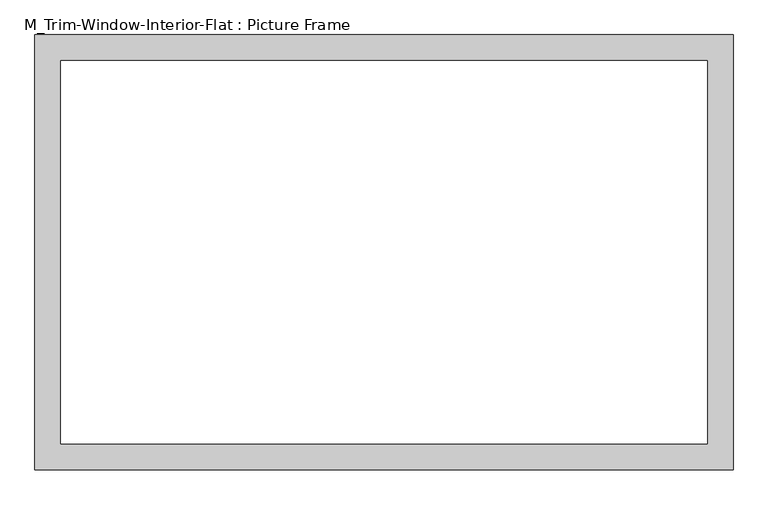
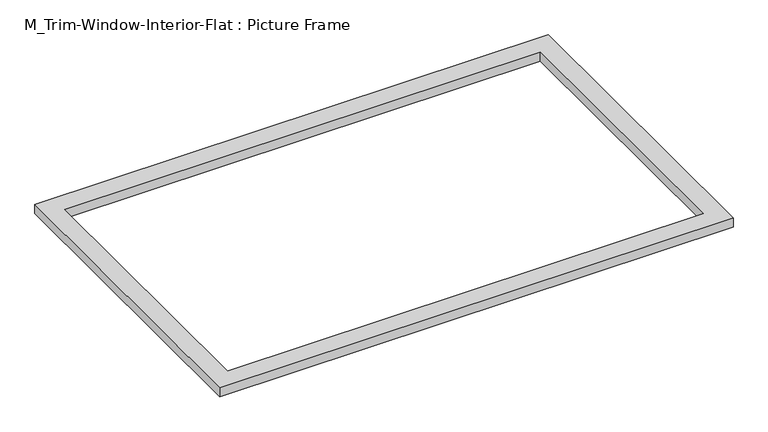
"""IFC4 building model written with IfcOpenShell, lengths in millimetres: proxy geometry, M_Trim-Window-Interior-Flat : Picture Frame."""

from ifc_helpers import new_model, si_unit, origin, origin_with_axes, place, context, project, spatial, polyline, outline, extrude, source, transform, mapped, element, save


def m_trim_window_interior_flat_picture_frame_7d8195fd(model_context):
    return source(origin(), model_context, "Body", "SweptSolid", [
        extrude(outline(polyline([(809.3, 47.3), (809.3, -961.7), (-809.3, -961.7), (-809.3, 47.3), (809.3, 47.3)]), holes=[polyline([(749.3, -12.7), (-749.3, -12.7), (-749.3, -901.7), (749.3, -901.7), (749.3, -12.7)])]), origin_with_axes(), (0.0, 0.0, 1.0), 30.0),
    ])


if __name__ == "__main__":
    model = new_model("IFC4")
    model_context = context("Model", 3, world=origin())
    ifc_project = project(units=[si_unit("LENGTHUNIT", "METRE", prefix="MILLI")], contexts=[model_context])
    site = spatial("IfcSite", under=ifc_project)
    building = spatial("IfcBuilding", under=site)
    placement = place(None, origin())
    m_trim_window_interior_flat_picture_frame_shape = m_trim_window_interior_flat_picture_frame_7d8195fd(model_context)
    element("IfcBuildingElementProxy", 1, Name="M_Trim-Window-Interior-Flat : Picture Frame", ObjectType="M_Trim-Window-Interior-Flat : Picture Frame", at=placement, inside=building, context=model_context, shape_type="MappedRepresentation", body=[
        mapped(m_trim_window_interior_flat_picture_frame_shape, transform((0.0, 0.0, 0.0), x_axis=(1.0, 0.0, 0.0), y_axis=(0.0, 1.0, 0.0), z_axis=(0.0, 0.0, 1.0))),
    ])
    save(model, "model.ifc")

# Revit data of these elements
# Type "M_Trim-Window-Interior-Flat : Picture Frame"
#   Trim Thickness_Picture Frame = 0' - 1.1811"
#   Trim Width = 0' - 2.3622"
#   Trim Thickness_with Sill = 0' - 0.7874"
#   Sill Thickness = 0' - 1.1811"
#   Opening Width [instance default] = 1' - 11.62205"
#   Opening Height [instance default] = 2' - 11.43307"
#   Default Elevation = 3' - 11.24409"
#   Sill = no
#   Picture Frame = yes
#   Trim Material [instance default] = none
# Element 1 (IfcBuildingElementProxy, "M_Trim-Window-Interior-Flat : Picture Frame")
#   Opening Width = 5' - 0"
#   Opening Height = 3' - 0"
#   Trim Material = Wood - Stained
#   Materials on its faces: "Wood - Stained"
# Materials
#   "Wood - Stained": class "Wood", colour RGB 224 178 126, transparency 0, Cost = 0
